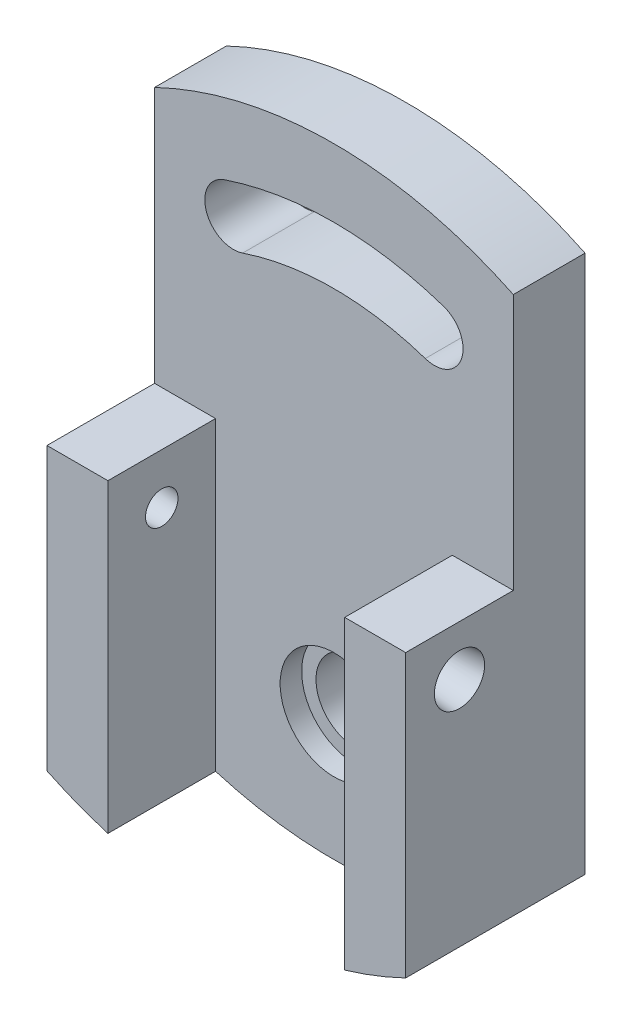
ISO-10303-21;
HEADER;
FILE_DESCRIPTION(('STEP AP214'),'2;1');
FILE_NAME('part.step','',(''),(''),'','','');
FILE_SCHEMA(('AUTOMOTIVE_DESIGN { 1 0 10303 214 1 1 1 1 }'));
ENDSEC;
DATA;
#1=APPLICATION_CONTEXT('core data for automotive mechanical design processes');
#2=APPLICATION_PROTOCOL_DEFINITION('international standard','automotive_design',2000,#1);
#3=PRODUCT_CONTEXT('',#1,'mechanical');
#4=PRODUCT('Part','Part','',(#3));
#5=PRODUCT_RELATED_PRODUCT_CATEGORY('part','',(#4));
#6=PRODUCT_DEFINITION_FORMATION('','',#4);
#7=PRODUCT_DEFINITION_CONTEXT('part definition',#1,'design');
#8=PRODUCT_DEFINITION('design','',#6,#7);
#9=PRODUCT_DEFINITION_SHAPE('','',#8);
#10=(LENGTH_UNIT() NAMED_UNIT(*) SI_UNIT(.MILLI.,.METRE.));
#11=(NAMED_UNIT(*) PLANE_ANGLE_UNIT() SI_UNIT($,.RADIAN.));
#12=(NAMED_UNIT(*) SI_UNIT($,.STERADIAN.) SOLID_ANGLE_UNIT());
#13=UNCERTAINTY_MEASURE_WITH_UNIT(LENGTH_MEASURE(1.E-05),#10,'distance_accuracy_value','');
#14=(GEOMETRIC_REPRESENTATION_CONTEXT(3) GLOBAL_UNCERTAINTY_ASSIGNED_CONTEXT((#13)) GLOBAL_UNIT_ASSIGNED_CONTEXT((#10,
#11,#12)) REPRESENTATION_CONTEXT('',''));
#15=CARTESIAN_POINT('',(0.,0.,0.));
#16=DIRECTION('',(0.,0.,1.));
#17=DIRECTION('',(1.,0.,0.));
#18=AXIS2_PLACEMENT_3D('',#15,#16,#17);
#19=CARTESIAN_POINT('',(0.,17.1231517720798,10.));
#20=DIRECTION('',(0.,0.,1.));
#21=DIRECTION('',(1.,0.,0.));
#22=AXIS2_PLACEMENT_3D('',#19,#20,#21);
#23=PLANE('',#22);
#24=CARTESIAN_POINT('',(28.,43.4266144584568,10.));
#25=DIRECTION('',(0.,0.,1.));
#26=DIRECTION('',(1.,0.,0.));
#27=AXIS2_PLACEMENT_3D('',#24,#25,#26);
#28=CIRCLE('',#27,8.00000000000001);
#29=CARTESIAN_POINT('',(25.4545454545455,35.8423767804153,10.));
#30=VERTEX_POINT('',#29);
#31=CARTESIAN_POINT('',(30.5454545454546,51.0108521364984,10.));
#32=VERTEX_POINT('',#31);
#33=EDGE_CURVE('E197',#30,#32,#28,.T.);
#34=ORIENTED_EDGE('',*,*,#33,.F.);
#35=CARTESIAN_POINT('',(0.,-40.,10.));
#36=DIRECTION('',(0.,0.,-1.));
#37=DIRECTION('',(1.,0.,0.));
#38=AXIS2_PLACEMENT_3D('',#35,#36,#37);
#39=CIRCLE('',#38,80.);
#40=CARTESIAN_POINT('',(-25.4545454545455,35.8423767804153,10.));
#41=VERTEX_POINT('',#40);
#42=EDGE_CURVE('E201',#41,#30,#39,.T.);
#43=ORIENTED_EDGE('',*,*,#42,.F.);
#44=CARTESIAN_POINT('',(-28.,43.4266144584568,10.));
#45=DIRECTION('',(0.,0.,1.));
#46=DIRECTION('',(1.,0.,0.));
#47=AXIS2_PLACEMENT_3D('',#44,#45,#46);
#48=CIRCLE('',#47,8.00000000000001);
#49=CARTESIAN_POINT('',(-30.5454545454545,51.0108521364984,10.));
#50=VERTEX_POINT('',#49);
#51=EDGE_CURVE('E213',#50,#41,#48,.T.);
#52=ORIENTED_EDGE('',*,*,#51,.F.);
#53=CARTESIAN_POINT('',(0.,-40.,10.));
#54=DIRECTION('',(0.,0.,1.));
#55=DIRECTION('',(1.,0.,0.));
#56=AXIS2_PLACEMENT_3D('',#53,#54,#55);
#57=CIRCLE('',#56,96.);
#58=EDGE_CURVE('E215',#32,#50,#57,.T.);
#59=ORIENTED_EDGE('',*,*,#58,.F.);
#60=EDGE_LOOP('',(#34,#43,#52,#59));
#61=FACE_BOUND('',#60,.T.);
#62=CARTESIAN_POINT('',(0.,-62.8768482279202,10.));
#63=DIRECTION('',(0.,0.,1.));
#64=DIRECTION('',(1.,0.,0.));
#65=AXIS2_PLACEMENT_3D('',#62,#63,#64);
#66=CIRCLE('',#65,15.);
#67=CARTESIAN_POINT('',(15.,-62.8768482279202,10.));
#68=VERTEX_POINT('',#67);
#69=EDGE_CURVE('E236',#68,#68,#66,.T.);
#70=ORIENTED_EDGE('',*,*,#69,.F.);
#71=EDGE_LOOP('',(#70));
#72=FACE_BOUND('',#71,.T.);
#73=DIRECTION('',(0.,-1.,0.));
#74=VECTOR('',#73,1.);
#75=CARTESIAN_POINT('',(33.,0.,10.));
#76=LINE('',#75,#74);
#77=CARTESIAN_POINT('',(33.,-7.87684822792019,10.));
#78=VERTEX_POINT('',#77);
#79=CARTESIAN_POINT('',(33.,-93.0403630592835,10.));
#80=VERTEX_POINT('',#79);
#81=EDGE_CURVE('E58',#78,#80,#76,.T.);
#82=ORIENTED_EDGE('',*,*,#81,.F.);
#83=DIRECTION('',(-1.,0.,0.));
#84=VECTOR('',#83,1.);
#85=CARTESIAN_POINT('',(0.,-7.87684822792019,10.));
#86=LINE('',#85,#84);
#87=CARTESIAN_POINT('',(50.,-7.87684822792019,10.));
#88=VERTEX_POINT('',#87);
#89=EDGE_CURVE('E317',#88,#78,#86,.T.);
#90=ORIENTED_EDGE('',*,*,#89,.F.);
#91=DIRECTION('',(0.,1.,0.));
#92=VECTOR('',#91,1.);
#93=CARTESIAN_POINT('',(50.,-86.4384241139601,10.));
#94=LINE('',#93,#92);
#95=CARTESIAN_POINT('',(50.,63.5615758860399,10.));
#96=VERTEX_POINT('',#95);
#97=EDGE_CURVE('E170',#88,#96,#94,.T.);
#98=ORIENTED_EDGE('',*,*,#97,.T.);
#99=CARTESIAN_POINT('',(0.,-40.,10.));
#100=DIRECTION('',(0.,0.,1.));
#101=DIRECTION('',(-1.,0.,0.));
#102=AXIS2_PLACEMENT_3D('',#99,#100,#101);
#103=CIRCLE('',#102,115.);
#104=CARTESIAN_POINT('',(-50.,63.5615758860399,10.));
#105=VERTEX_POINT('',#104);
#106=EDGE_CURVE('E245',#96,#105,#103,.T.);
#107=ORIENTED_EDGE('',*,*,#106,.T.);
#108=DIRECTION('',(0.,-1.,0.));
#109=VECTOR('',#108,1.);
#110=CARTESIAN_POINT('',(-50.,-86.4384241139601,10.));
#111=LINE('',#110,#109);
#112=CARTESIAN_POINT('',(-50.,-7.87684822792019,10.));
#113=VERTEX_POINT('',#112);
#114=EDGE_CURVE('E242',#105,#113,#111,.T.);
#115=ORIENTED_EDGE('',*,*,#114,.T.);
#116=DIRECTION('',(1.,0.,0.));
#117=VECTOR('',#116,1.);
#118=CARTESIAN_POINT('',(0.,-7.87684822792019,10.));
#119=LINE('',#118,#117);
#120=CARTESIAN_POINT('',(-33.,-7.87684822792019,10.));
#121=VERTEX_POINT('',#120);
#122=EDGE_CURVE('E167',#113,#121,#119,.T.);
#123=ORIENTED_EDGE('',*,*,#122,.T.);
#124=DIRECTION('',(0.,-1.,0.));
#125=VECTOR('',#124,1.);
#126=CARTESIAN_POINT('',(-33.,0.,10.));
#127=LINE('',#126,#125);
#128=CARTESIAN_POINT('',(-33.,-93.0403630592835,10.));
#129=VERTEX_POINT('',#128);
#130=EDGE_CURVE('E166',#121,#129,#127,.T.);
#131=ORIENTED_EDGE('',*,*,#130,.T.);
#132=CARTESIAN_POINT('',(0.,17.1231517720798,10.));
#133=DIRECTION('',(0.,0.,1.));
#134=DIRECTION('',(1.,0.,0.));
#135=AXIS2_PLACEMENT_3D('',#132,#133,#134);
#136=CIRCLE('',#135,115.);
#137=EDGE_CURVE('E63',#129,#80,#136,.T.);
#138=ORIENTED_EDGE('',*,*,#137,.T.);
#139=EDGE_LOOP('',(#82,#90,#98,#107,#115,#123,#131,#138));
#140=FACE_BOUND('',#139,.T.);
#141=ADVANCED_FACE('F43',(#61,#72,#140),#23,.T.);
#142=CARTESIAN_POINT('',(0.,17.1231517720798,10.));
#143=DIRECTION('',(0.,0.,-1.));
#144=DIRECTION('',(-1.,0.,0.));
#145=AXIS2_PLACEMENT_3D('',#142,#143,#144);
#146=CYLINDRICAL_SURFACE('',#145,115.);
#147=CARTESIAN_POINT('',(0.,17.1231517720798,-10.));
#148=DIRECTION('',(0.,0.,1.));
#149=DIRECTION('',(1.,0.,0.));
#150=AXIS2_PLACEMENT_3D('',#147,#148,#149);
#151=CIRCLE('',#150,115.);
#152=CARTESIAN_POINT('',(-50.,-86.4384241139601,-10.));
#153=VERTEX_POINT('',#152);
#154=CARTESIAN_POINT('',(50.,-86.4384241139601,-10.));
#155=VERTEX_POINT('',#154);
#156=EDGE_CURVE('E232',#153,#155,#151,.T.);
#157=ORIENTED_EDGE('',*,*,#156,.T.);
#158=DIRECTION('',(0.,0.,-1.));
#159=VECTOR('',#158,1.);
#160=CARTESIAN_POINT('',(50.,-86.4384241139601,10.));
#161=LINE('',#160,#159);
#162=CARTESIAN_POINT('',(50.,-86.4384241139601,40.));
#163=VERTEX_POINT('',#162);
#164=EDGE_CURVE('E12',#163,#155,#161,.T.);
#165=ORIENTED_EDGE('',*,*,#164,.F.);
#166=CARTESIAN_POINT('',(0.,17.1231517720798,40.));
#167=DIRECTION('',(0.,0.,1.));
#168=DIRECTION('',(1.,0.,0.));
#169=AXIS2_PLACEMENT_3D('',#166,#167,#168);
#170=CIRCLE('',#169,115.);
#171=CARTESIAN_POINT('',(33.,-93.0403630592835,40.));
#172=VERTEX_POINT('',#171);
#173=EDGE_CURVE('E162',#172,#163,#170,.T.);
#174=ORIENTED_EDGE('',*,*,#173,.F.);
#175=DIRECTION('',(0.,0.,-1.));
#176=VECTOR('',#175,1.);
#177=CARTESIAN_POINT('',(33.,-93.0403630592835,40.));
#178=LINE('',#177,#176);
#179=EDGE_CURVE('E175',#172,#80,#178,.T.);
#180=ORIENTED_EDGE('',*,*,#179,.T.);
#181=ORIENTED_EDGE('',*,*,#137,.F.);
#182=DIRECTION('',(0.,0.,-1.));
#183=VECTOR('',#182,1.);
#184=CARTESIAN_POINT('',(-33.,-93.0403630592835,40.));
#185=LINE('',#184,#183);
#186=CARTESIAN_POINT('',(-33.,-93.0403630592835,40.));
#187=VERTEX_POINT('',#186);
#188=EDGE_CURVE('E187',#187,#129,#185,.T.);
#189=ORIENTED_EDGE('',*,*,#188,.F.);
#190=CARTESIAN_POINT('',(0.,17.1231517720798,40.));
#191=DIRECTION('',(0.,0.,1.));
#192=DIRECTION('',(1.,0.,0.));
#193=AXIS2_PLACEMENT_3D('',#190,#191,#192);
#194=CIRCLE('',#193,115.);
#195=CARTESIAN_POINT('',(-50.,-86.4384241139601,40.));
#196=VERTEX_POINT('',#195);
#197=EDGE_CURVE('E184',#196,#187,#194,.T.);
#198=ORIENTED_EDGE('',*,*,#197,.F.);
#199=DIRECTION('',(0.,0.,-1.));
#200=VECTOR('',#199,1.);
#201=CARTESIAN_POINT('',(-50.,-86.4384241139601,10.));
#202=LINE('',#201,#200);
#203=EDGE_CURVE('E250',#196,#153,#202,.T.);
#204=ORIENTED_EDGE('',*,*,#203,.T.);
#205=EDGE_LOOP('',(#157,#165,#174,#180,#181,#189,#198,#204));
#206=FACE_BOUND('',#205,.T.);
#207=ADVANCED_FACE('F44',(#206),#146,.T.);
#208=CARTESIAN_POINT('',(50.,-86.4384241139601,10.));
#209=DIRECTION('',(-1.,0.,0.));
#210=DIRECTION('',(0.,0.,1.));
#211=AXIS2_PLACEMENT_3D('',#208,#209,#210);
#212=PLANE('',#211);
#213=CARTESIAN_POINT('',(50.,-21.8768482279202,25.));
#214=DIRECTION('',(1.,0.,0.));
#215=DIRECTION('',(0.,0.,-1.));
#216=AXIS2_PLACEMENT_3D('',#213,#214,#215);
#217=CIRCLE('',#216,7.);
#218=CARTESIAN_POINT('',(50.,-18.0410436799808,30.8554763657628));
#219=VERTEX_POINT('',#218);
#220=EDGE_CURVE('E310',#219,#219,#217,.T.);
#221=ORIENTED_EDGE('',*,*,#220,.F.);
#222=EDGE_LOOP('',(#221));
#223=FACE_BOUND('',#222,.T.);
#224=DIRECTION('',(0.,1.,0.));
#225=VECTOR('',#224,1.);
#226=CARTESIAN_POINT('',(50.,-86.4384241139601,-10.));
#227=LINE('',#226,#225);
#228=CARTESIAN_POINT('',(50.,63.5615758860399,-10.));
#229=VERTEX_POINT('',#228);
#230=EDGE_CURVE('E249',#155,#229,#227,.T.);
#231=ORIENTED_EDGE('',*,*,#230,.T.);
#232=DIRECTION('',(0.,0.,-1.));
#233=VECTOR('',#232,1.);
#234=CARTESIAN_POINT('',(50.,63.5615758860399,10.));
#235=LINE('',#234,#233);
#236=EDGE_CURVE('E55',#96,#229,#235,.T.);
#237=ORIENTED_EDGE('',*,*,#236,.F.);
#238=ORIENTED_EDGE('',*,*,#97,.F.);
#239=DIRECTION('',(0.,0.,-1.));
#240=VECTOR('',#239,1.);
#241=CARTESIAN_POINT('',(50.,-7.87684822792019,40.));
#242=LINE('',#241,#240);
#243=CARTESIAN_POINT('',(50.,-7.87684822792019,40.));
#244=VERTEX_POINT('',#243);
#245=EDGE_CURVE('E148',#244,#88,#242,.T.);
#246=ORIENTED_EDGE('',*,*,#245,.F.);
#247=DIRECTION('',(0.,1.,0.));
#248=VECTOR('',#247,1.);
#249=CARTESIAN_POINT('',(50.,0.,40.));
#250=LINE('',#249,#248);
#251=EDGE_CURVE('E156',#163,#244,#250,.T.);
#252=ORIENTED_EDGE('',*,*,#251,.F.);
#253=ORIENTED_EDGE('',*,*,#164,.T.);
#254=EDGE_LOOP('',(#231,#237,#238,#246,#252,#253));
#255=FACE_BOUND('',#254,.T.);
#256=ADVANCED_FACE('F164',(#223,#255),#212,.F.);
#257=CARTESIAN_POINT('',(0.,-40.,10.));
#258=DIRECTION('',(0.,0.,-1.));
#259=DIRECTION('',(-1.,0.,0.));
#260=AXIS2_PLACEMENT_3D('',#257,#258,#259);
#261=CYLINDRICAL_SURFACE('',#260,115.);
#262=CARTESIAN_POINT('',(0.,-40.,-10.));
#263=DIRECTION('',(0.,0.,1.));
#264=DIRECTION('',(-1.,0.,0.));
#265=AXIS2_PLACEMENT_3D('',#262,#263,#264);
#266=CIRCLE('',#265,115.);
#267=CARTESIAN_POINT('',(-50.,63.5615758860399,-10.));
#268=VERTEX_POINT('',#267);
#269=EDGE_CURVE('E255',#229,#268,#266,.T.);
#270=ORIENTED_EDGE('',*,*,#269,.T.);
#271=DIRECTION('',(0.,0.,-1.));
#272=VECTOR('',#271,1.);
#273=CARTESIAN_POINT('',(-50.,63.5615758860399,10.));
#274=LINE('',#273,#272);
#275=EDGE_CURVE('E260',#105,#268,#274,.T.);
#276=ORIENTED_EDGE('',*,*,#275,.F.);
#277=ORIENTED_EDGE('',*,*,#106,.F.);
#278=ORIENTED_EDGE('',*,*,#236,.T.);
#279=EDGE_LOOP('',(#270,#276,#277,#278));
#280=FACE_BOUND('',#279,.T.);
#281=ADVANCED_FACE('F298',(#280),#261,.T.);
#282=CARTESIAN_POINT('',(-50.,-86.4384241139601,10.));
#283=DIRECTION('',(1.,0.,0.));
#284=DIRECTION('',(0.,0.,-1.));
#285=AXIS2_PLACEMENT_3D('',#282,#283,#284);
#286=PLANE('',#285);
#287=CARTESIAN_POINT('',(-50.,-21.8768482279202,25.));
#288=DIRECTION('',(-1.,0.,0.));
#289=DIRECTION('',(0.,0.,1.));
#290=AXIS2_PLACEMENT_3D('',#287,#288,#289);
#291=CIRCLE('',#290,6.);
#292=CARTESIAN_POINT('',(-50.,-27.8608007953017,25.4385335464111));
#293=VERTEX_POINT('',#292);
#294=EDGE_CURVE('E307',#293,#293,#291,.T.);
#295=ORIENTED_EDGE('',*,*,#294,.F.);
#296=EDGE_LOOP('',(#295));
#297=FACE_BOUND('',#296,.T.);
#298=DIRECTION('',(0.,-1.,0.));
#299=VECTOR('',#298,1.);
#300=CARTESIAN_POINT('',(-50.,-86.4384241139601,-10.));
#301=LINE('',#300,#299);
#302=EDGE_CURVE('E239',#268,#153,#301,.T.);
#303=ORIENTED_EDGE('',*,*,#302,.T.);
#304=ORIENTED_EDGE('',*,*,#203,.F.);
#305=DIRECTION('',(0.,-1.,0.));
#306=VECTOR('',#305,1.);
#307=CARTESIAN_POINT('',(-50.,0.,40.));
#308=LINE('',#307,#306);
#309=CARTESIAN_POINT('',(-50.,-7.87684822792019,40.));
#310=VERTEX_POINT('',#309);
#311=EDGE_CURVE('E185',#310,#196,#308,.T.);
#312=ORIENTED_EDGE('',*,*,#311,.F.);
#313=DIRECTION('',(0.,0.,-1.));
#314=VECTOR('',#313,1.);
#315=CARTESIAN_POINT('',(-50.,-7.87684822792019,40.));
#316=LINE('',#315,#314);
#317=EDGE_CURVE('E192',#310,#113,#316,.T.);
#318=ORIENTED_EDGE('',*,*,#317,.T.);
#319=ORIENTED_EDGE('',*,*,#114,.F.);
#320=ORIENTED_EDGE('',*,*,#275,.T.);
#321=EDGE_LOOP('',(#303,#304,#312,#318,#319,#320));
#322=FACE_BOUND('',#321,.T.);
#323=ADVANCED_FACE('F292',(#297,#322),#286,.F.);
#324=CARTESIAN_POINT('',(0.,17.1231517720798,-10.));
#325=DIRECTION('',(0.,0.,1.));
#326=DIRECTION('',(1.,0.,0.));
#327=AXIS2_PLACEMENT_3D('',#324,#325,#326);
#328=PLANE('',#327);
#329=CARTESIAN_POINT('',(0.,-40.,-10.));
#330=DIRECTION('',(0.,0.,-1.));
#331=DIRECTION('',(1.,0.,0.));
#332=AXIS2_PLACEMENT_3D('',#329,#330,#331);
#333=CIRCLE('',#332,80.);
#334=CARTESIAN_POINT('',(-25.4545454545455,35.8423767804153,-10.));
#335=VERTEX_POINT('',#334);
#336=CARTESIAN_POINT('',(25.4545454545455,35.8423767804153,-10.));
#337=VERTEX_POINT('',#336);
#338=EDGE_CURVE('E210',#335,#337,#333,.T.);
#339=ORIENTED_EDGE('',*,*,#338,.T.);
#340=CARTESIAN_POINT('',(28.,43.4266144584568,-10.));
#341=DIRECTION('',(0.,0.,1.));
#342=DIRECTION('',(1.,0.,0.));
#343=AXIS2_PLACEMENT_3D('',#340,#341,#342);
#344=CIRCLE('',#343,8.00000000000001);
#345=CARTESIAN_POINT('',(30.5454545454546,51.0108521364984,-10.));
#346=VERTEX_POINT('',#345);
#347=EDGE_CURVE('E200',#337,#346,#344,.T.);
#348=ORIENTED_EDGE('',*,*,#347,.T.);
#349=CARTESIAN_POINT('',(0.,-40.,-10.));
#350=DIRECTION('',(0.,0.,1.));
#351=DIRECTION('',(1.,0.,0.));
#352=AXIS2_PLACEMENT_3D('',#349,#350,#351);
#353=CIRCLE('',#352,96.);
#354=CARTESIAN_POINT('',(-30.5454545454545,51.0108521364984,-10.));
#355=VERTEX_POINT('',#354);
#356=EDGE_CURVE('E198',#346,#355,#353,.T.);
#357=ORIENTED_EDGE('',*,*,#356,.T.);
#358=CARTESIAN_POINT('',(-28.,43.4266144584568,-10.));
#359=DIRECTION('',(0.,0.,1.));
#360=DIRECTION('',(1.,0.,0.));
#361=AXIS2_PLACEMENT_3D('',#358,#359,#360);
#362=CIRCLE('',#361,8.00000000000001);
#363=EDGE_CURVE('E203',#355,#335,#362,.T.);
#364=ORIENTED_EDGE('',*,*,#363,.T.);
#365=EDGE_LOOP('',(#339,#348,#357,#364));
#366=FACE_BOUND('',#365,.T.);
#367=CARTESIAN_POINT('',(0.,-62.8768482279202,-10.));
#368=DIRECTION('',(0.,0.,1.));
#369=DIRECTION('',(1.,0.,0.));
#370=AXIS2_PLACEMENT_3D('',#367,#368,#369);
#371=CIRCLE('',#370,11.);
#372=CARTESIAN_POINT('',(11.,-62.8768482279202,-10.));
#373=VERTEX_POINT('',#372);
#374=EDGE_CURVE('E225',#373,#373,#371,.T.);
#375=ORIENTED_EDGE('',*,*,#374,.T.);
#376=EDGE_LOOP('',(#375));
#377=FACE_BOUND('',#376,.T.);
#378=ORIENTED_EDGE('',*,*,#156,.F.);
#379=ORIENTED_EDGE('',*,*,#302,.F.);
#380=ORIENTED_EDGE('',*,*,#269,.F.);
#381=ORIENTED_EDGE('',*,*,#230,.F.);
#382=EDGE_LOOP('',(#378,#379,#380,#381));
#383=FACE_BOUND('',#382,.T.);
#384=ADVANCED_FACE('F277',(#366,#377,#383),#328,.F.);
#385=CARTESIAN_POINT('',(0.,-62.8768482279202,4.));
#386=DIRECTION('',(0.,0.,1.));
#387=DIRECTION('',(1.,0.,0.));
#388=AXIS2_PLACEMENT_3D('',#385,#386,#387);
#389=CYLINDRICAL_SURFACE('',#388,15.);
#390=CARTESIAN_POINT('',(0.,-62.8768482279202,4.));
#391=DIRECTION('',(0.,0.,1.));
#392=DIRECTION('',(1.,0.,0.));
#393=AXIS2_PLACEMENT_3D('',#390,#391,#392);
#394=CIRCLE('',#393,15.);
#395=CARTESIAN_POINT('',(15.,-62.8768482279202,4.));
#396=VERTEX_POINT('',#395);
#397=EDGE_CURVE('E235',#396,#396,#394,.T.);
#398=ORIENTED_EDGE('',*,*,#397,.F.);
#399=EDGE_LOOP('',(#398));
#400=FACE_BOUND('',#399,.T.);
#401=ORIENTED_EDGE('',*,*,#69,.T.);
#402=EDGE_LOOP('',(#401));
#403=FACE_BOUND('',#402,.T.);
#404=ADVANCED_FACE('F269',(#400,#403),#389,.F.);
#405=CARTESIAN_POINT('',(0.,-62.8768482279202,4.));
#406=DIRECTION('',(0.,0.,1.));
#407=DIRECTION('',(1.,0.,0.));
#408=AXIS2_PLACEMENT_3D('',#405,#406,#407);
#409=PLANE('',#408);
#410=CARTESIAN_POINT('',(0.,-62.8768482279202,4.));
#411=DIRECTION('',(0.,0.,1.));
#412=DIRECTION('',(1.,0.,0.));
#413=AXIS2_PLACEMENT_3D('',#410,#411,#412);
#414=CIRCLE('',#413,11.);
#415=CARTESIAN_POINT('',(11.,-62.8768482279202,4.));
#416=VERTEX_POINT('',#415);
#417=EDGE_CURVE('E233',#416,#416,#414,.T.);
#418=ORIENTED_EDGE('',*,*,#417,.F.);
#419=EDGE_LOOP('',(#418));
#420=FACE_BOUND('',#419,.T.);
#421=ORIENTED_EDGE('',*,*,#397,.T.);
#422=EDGE_LOOP('',(#421));
#423=FACE_BOUND('',#422,.T.);
#424=ADVANCED_FACE('F270',(#420,#423),#409,.T.);
#425=CARTESIAN_POINT('',(0.,-62.8768482279202,-10.));
#426=DIRECTION('',(0.,0.,1.));
#427=DIRECTION('',(1.,0.,0.));
#428=AXIS2_PLACEMENT_3D('',#425,#426,#427);
#429=CYLINDRICAL_SURFACE('',#428,11.);
#430=ORIENTED_EDGE('',*,*,#417,.T.);
#431=EDGE_LOOP('',(#430));
#432=FACE_BOUND('',#431,.T.);
#433=ORIENTED_EDGE('',*,*,#374,.F.);
#434=EDGE_LOOP('',(#433));
#435=FACE_BOUND('',#434,.T.);
#436=ADVANCED_FACE('F261',(#432,#435),#429,.F.);
#437=CARTESIAN_POINT('',(28.,43.4266144584568,-10.));
#438=DIRECTION('',(0.,0.,1.));
#439=DIRECTION('',(1.,0.,0.));
#440=AXIS2_PLACEMENT_3D('',#437,#438,#439);
#441=CYLINDRICAL_SURFACE('',#440,8.00000000000001);
#442=ORIENTED_EDGE('',*,*,#33,.T.);
#443=DIRECTION('',(0.,0.,1.));
#444=VECTOR('',#443,1.);
#445=CARTESIAN_POINT('',(30.5454545454546,51.0108521364984,-10.));
#446=LINE('',#445,#444);
#447=EDGE_CURVE('E208',#346,#32,#446,.T.);
#448=ORIENTED_EDGE('',*,*,#447,.F.);
#449=ORIENTED_EDGE('',*,*,#347,.F.);
#450=DIRECTION('',(0.,0.,1.));
#451=VECTOR('',#450,1.);
#452=CARTESIAN_POINT('',(25.4545454545455,35.8423767804153,-10.));
#453=LINE('',#452,#451);
#454=EDGE_CURVE('E218',#337,#30,#453,.T.);
#455=ORIENTED_EDGE('',*,*,#454,.T.);
#456=EDGE_LOOP('',(#442,#448,#449,#455));
#457=FACE_BOUND('',#456,.T.);
#458=ADVANCED_FACE('F358',(#457),#441,.F.);
#459=CARTESIAN_POINT('',(0.,-40.,-10.));
#460=DIRECTION('',(0.,0.,1.));
#461=DIRECTION('',(1.,0.,0.));
#462=AXIS2_PLACEMENT_3D('',#459,#460,#461);
#463=CYLINDRICAL_SURFACE('',#462,80.);
#464=ORIENTED_EDGE('',*,*,#42,.T.);
#465=ORIENTED_EDGE('',*,*,#454,.F.);
#466=ORIENTED_EDGE('',*,*,#338,.F.);
#467=DIRECTION('',(0.,0.,1.));
#468=VECTOR('',#467,1.);
#469=CARTESIAN_POINT('',(-25.4545454545455,35.8423767804153,-10.));
#470=LINE('',#469,#468);
#471=EDGE_CURVE('E222',#335,#41,#470,.T.);
#472=ORIENTED_EDGE('',*,*,#471,.T.);
#473=EDGE_LOOP('',(#464,#465,#466,#472));
#474=FACE_BOUND('',#473,.T.);
#475=ADVANCED_FACE('F355',(#474),#463,.T.);
#476=CARTESIAN_POINT('',(-28.,43.4266144584568,-10.));
#477=DIRECTION('',(0.,0.,1.));
#478=DIRECTION('',(1.,0.,0.));
#479=AXIS2_PLACEMENT_3D('',#476,#477,#478);
#480=CYLINDRICAL_SURFACE('',#479,8.00000000000001);
#481=ORIENTED_EDGE('',*,*,#51,.T.);
#482=ORIENTED_EDGE('',*,*,#471,.F.);
#483=ORIENTED_EDGE('',*,*,#363,.F.);
#484=DIRECTION('',(0.,0.,1.));
#485=VECTOR('',#484,1.);
#486=CARTESIAN_POINT('',(-30.5454545454545,51.0108521364984,-10.));
#487=LINE('',#486,#485);
#488=EDGE_CURVE('E224',#355,#50,#487,.T.);
#489=ORIENTED_EDGE('',*,*,#488,.T.);
#490=EDGE_LOOP('',(#481,#482,#483,#489));
#491=FACE_BOUND('',#490,.T.);
#492=ADVANCED_FACE('F354',(#491),#480,.F.);
#493=CARTESIAN_POINT('',(0.,-40.,-10.));
#494=DIRECTION('',(0.,0.,1.));
#495=DIRECTION('',(1.,0.,0.));
#496=AXIS2_PLACEMENT_3D('',#493,#494,#495);
#497=CYLINDRICAL_SURFACE('',#496,96.);
#498=ORIENTED_EDGE('',*,*,#58,.T.);
#499=ORIENTED_EDGE('',*,*,#488,.F.);
#500=ORIENTED_EDGE('',*,*,#356,.F.);
#501=ORIENTED_EDGE('',*,*,#447,.T.);
#502=EDGE_LOOP('',(#498,#499,#500,#501));
#503=FACE_BOUND('',#502,.T.);
#504=ADVANCED_FACE('F348',(#503),#497,.F.);
#505=CARTESIAN_POINT('',(-33.,0.,40.));
#506=DIRECTION('',(1.,0.,0.));
#507=DIRECTION('',(0.,1.,0.));
#508=AXIS2_PLACEMENT_3D('',#505,#506,#507);
#509=PLANE('',#508);
#510=CARTESIAN_POINT('',(-33.,-21.8768482279202,25.));
#511=DIRECTION('',(-1.,0.,0.));
#512=DIRECTION('',(0.,0.,1.));
#513=AXIS2_PLACEMENT_3D('',#510,#511,#512);
#514=CIRCLE('',#513,4.52368501413102);
#515=CARTESIAN_POINT('',(-33.,-26.1914420856972,26.3594138257009));
#516=VERTEX_POINT('',#515);
#517=EDGE_CURVE('E313',#516,#516,#514,.F.);
#518=ORIENTED_EDGE('',*,*,#517,.F.);
#519=EDGE_LOOP('',(#518));
#520=FACE_BOUND('',#519,.T.);
#521=ORIENTED_EDGE('',*,*,#130,.F.);
#522=DIRECTION('',(0.,0.,-1.));
#523=VECTOR('',#522,1.);
#524=CARTESIAN_POINT('',(-33.,-7.87684822792019,40.));
#525=LINE('',#524,#523);
#526=CARTESIAN_POINT('',(-33.,-7.87684822792019,40.));
#527=VERTEX_POINT('',#526);
#528=EDGE_CURVE('E194',#527,#121,#525,.T.);
#529=ORIENTED_EDGE('',*,*,#528,.F.);
#530=DIRECTION('',(0.,-1.,0.));
#531=VECTOR('',#530,1.);
#532=CARTESIAN_POINT('',(-33.,0.,40.));
#533=LINE('',#532,#531);
#534=EDGE_CURVE('E176',#527,#187,#533,.T.);
#535=ORIENTED_EDGE('',*,*,#534,.T.);
#536=ORIENTED_EDGE('',*,*,#188,.T.);
#537=EDGE_LOOP('',(#521,#529,#535,#536));
#538=FACE_BOUND('',#537,.T.);
#539=ADVANCED_FACE('F350',(#520,#538),#509,.T.);
#540=CARTESIAN_POINT('',(0.,-7.87684822792019,40.));
#541=DIRECTION('',(0.,1.,0.));
#542=DIRECTION('',(0.,0.,1.));
#543=AXIS2_PLACEMENT_3D('',#540,#541,#542);
#544=PLANE('',#543);
#545=ORIENTED_EDGE('',*,*,#122,.F.);
#546=ORIENTED_EDGE('',*,*,#317,.F.);
#547=DIRECTION('',(1.,0.,0.));
#548=VECTOR('',#547,1.);
#549=CARTESIAN_POINT('',(0.,-7.87684822792019,40.));
#550=LINE('',#549,#548);
#551=EDGE_CURVE('E177',#310,#527,#550,.T.);
#552=ORIENTED_EDGE('',*,*,#551,.T.);
#553=ORIENTED_EDGE('',*,*,#528,.T.);
#554=EDGE_LOOP('',(#545,#546,#552,#553));
#555=FACE_BOUND('',#554,.T.);
#556=ADVANCED_FACE('F344',(#555),#544,.T.);
#557=CARTESIAN_POINT('',(0.,0.,40.));
#558=DIRECTION('',(0.,0.,1.));
#559=DIRECTION('',(1.,0.,0.));
#560=AXIS2_PLACEMENT_3D('',#557,#558,#559);
#561=PLANE('',#560);
#562=ORIENTED_EDGE('',*,*,#534,.F.);
#563=ORIENTED_EDGE('',*,*,#551,.F.);
#564=ORIENTED_EDGE('',*,*,#311,.T.);
#565=ORIENTED_EDGE('',*,*,#197,.T.);
#566=EDGE_LOOP('',(#562,#563,#564,#565));
#567=FACE_BOUND('',#566,.T.);
#568=ADVANCED_FACE('F337',(#567),#561,.T.);
#569=CARTESIAN_POINT('',(0.,-7.87684822792019,40.));
#570=DIRECTION('',(0.,-1.,0.));
#571=DIRECTION('',(0.,0.,-1.));
#572=AXIS2_PLACEMENT_3D('',#569,#570,#571);
#573=PLANE('',#572);
#574=ORIENTED_EDGE('',*,*,#89,.T.);
#575=DIRECTION('',(0.,0.,-1.));
#576=VECTOR('',#575,1.);
#577=CARTESIAN_POINT('',(33.,-7.87684822792019,40.));
#578=LINE('',#577,#576);
#579=CARTESIAN_POINT('',(33.,-7.87684822792019,40.));
#580=VERTEX_POINT('',#579);
#581=EDGE_CURVE('E155',#580,#78,#578,.T.);
#582=ORIENTED_EDGE('',*,*,#581,.F.);
#583=DIRECTION('',(-1.,0.,0.));
#584=VECTOR('',#583,1.);
#585=CARTESIAN_POINT('',(0.,-7.87684822792019,40.));
#586=LINE('',#585,#584);
#587=EDGE_CURVE('E147',#244,#580,#586,.T.);
#588=ORIENTED_EDGE('',*,*,#587,.F.);
#589=ORIENTED_EDGE('',*,*,#245,.T.);
#590=EDGE_LOOP('',(#574,#582,#588,#589));
#591=FACE_BOUND('',#590,.T.);
#592=ADVANCED_FACE('F149',(#591),#573,.F.);
#593=CARTESIAN_POINT('',(33.,0.,40.));
#594=DIRECTION('',(1.,0.,0.));
#595=DIRECTION('',(0.,1.,0.));
#596=AXIS2_PLACEMENT_3D('',#593,#594,#595);
#597=PLANE('',#596);
#598=CARTESIAN_POINT('',(33.,-21.8768482279202,25.));
#599=DIRECTION('',(-1.,0.,0.));
#600=DIRECTION('',(0.,0.,1.));
#601=AXIS2_PLACEMENT_3D('',#598,#599,#600);
#602=CIRCLE('',#601,5.38922314504359);
#603=CARTESIAN_POINT('',(33.,-19.7104023895853,29.9345960864731));
#604=VERTEX_POINT('',#603);
#605=EDGE_CURVE('E50',#604,#604,#602,.F.);
#606=ORIENTED_EDGE('',*,*,#605,.T.);
#607=EDGE_LOOP('',(#606));
#608=FACE_BOUND('',#607,.T.);
#609=ORIENTED_EDGE('',*,*,#81,.T.);
#610=ORIENTED_EDGE('',*,*,#179,.F.);
#611=DIRECTION('',(0.,-1.,0.));
#612=VECTOR('',#611,1.);
#613=CARTESIAN_POINT('',(33.,0.,40.));
#614=LINE('',#613,#612);
#615=EDGE_CURVE('E153',#580,#172,#614,.T.);
#616=ORIENTED_EDGE('',*,*,#615,.F.);
#617=ORIENTED_EDGE('',*,*,#581,.T.);
#618=EDGE_LOOP('',(#609,#610,#616,#617));
#619=FACE_BOUND('',#618,.T.);
#620=ADVANCED_FACE('F323',(#608,#619),#597,.F.);
#621=CARTESIAN_POINT('',(0.,0.,40.));
#622=DIRECTION('',(0.,0.,1.));
#623=DIRECTION('',(1.,0.,0.));
#624=AXIS2_PLACEMENT_3D('',#621,#622,#623);
#625=PLANE('',#624);
#626=ORIENTED_EDGE('',*,*,#251,.T.);
#627=ORIENTED_EDGE('',*,*,#587,.T.);
#628=ORIENTED_EDGE('',*,*,#615,.T.);
#629=ORIENTED_EDGE('',*,*,#173,.T.);
#630=EDGE_LOOP('',(#626,#627,#628,#629));
#631=FACE_BOUND('',#630,.T.);
#632=ADVANCED_FACE('F159',(#631),#625,.T.);
#633=CARTESIAN_POINT('',(50.,-18.0410436799808,30.8554763657628));
#634=CARTESIAN_POINT('',(-50.,-27.8608007953017,25.4385335464111));
#635=CARTESIAN_POINT('',(50.,-6.33009094845508,23.183867269884));
#636=CARTESIAN_POINT('',(-50.,-26.9837337024795,37.4064386811742));
#637=CARTESIAN_POINT('',(50.,-14.0017000443339,11.4729145383583));
#638=CARTESIAN_POINT('',(-50.,-15.0158285677164,36.529371588352));
#639=CARTESIAN_POINT('',(50.,-25.7126527758596,19.1445236342372));
#640=CARTESIAN_POINT('',(-50.,-15.8928956605387,24.5614664535889));
#641=CARTESIAN_POINT('',(50.,-37.4236055073853,26.816132730116));
#642=CARTESIAN_POINT('',(-50.,-16.7699627533609,12.5935613188258));
#643=CARTESIAN_POINT('',(50.,-29.7519964115064,38.5270854616417));
#644=CARTESIAN_POINT('',(-50.,-28.737867888124,13.470628411648));
#645=CARTESIAN_POINT('',(50.,-18.0410436799808,30.8554763657628));
#646=CARTESIAN_POINT('',(-50.,-27.8608007953017,25.4385335464111));
#647=(BOUNDED_SURFACE() B_SPLINE_SURFACE(3,1,((#633,#634),(#635,#636),(#637,#638),(#639,#640),
(#641,#642),(#643,#644),(#645,#646)),.UNSPECIFIED.,.T.,.F.,.F.) B_SPLINE_SURFACE_WITH_KNOTS((4,
3,4),(2,2),(0.,0.5,1.),(0.,1.),
.UNSPECIFIED.) GEOMETRIC_REPRESENTATION_ITEM() RATIONAL_B_SPLINE_SURFACE(((1.,1.),
(0.333333333333333,0.333333333333333),(0.333333333333333,0.333333333333333),(1.,1.),
(0.333333333333333,0.333333333333333),(0.333333333333333,0.333333333333333),(1.,1.))) REPRESENTATION_ITEM('') SURFACE());
#648=CARTESIAN_POINT('',(50.,-18.0410436799808,30.8554763657628));
#649=CARTESIAN_POINT('',(49.8229166666667,-18.0584328332058,30.8458838628536));
#650=CARTESIAN_POINT('',(49.6458333333333,-18.0758219864309,30.8362913599443));
#651=CARTESIAN_POINT('',(49.2916666666667,-18.1106002928809,30.8171063541258));
#652=CARTESIAN_POINT('',(49.1145833333333,-18.127989446106,30.8075138512165));
#653=CARTESIAN_POINT('',(48.7604166666667,-18.1627677525561,30.788328845398));
#654=CARTESIAN_POINT('',(48.5833333333333,-18.1801569057811,30.7787363424887));
#655=CARTESIAN_POINT('',(48.2291666666667,-18.2149352122312,30.7595513366702));
#656=CARTESIAN_POINT('',(48.0520833333333,-18.2323243654563,30.7499588337609));
#657=CARTESIAN_POINT('',(47.6979166666667,-18.2671026719064,30.7307738279423));
#658=CARTESIAN_POINT('',(47.5208333333333,-18.2844918251314,30.7211813250331));
#659=CARTESIAN_POINT('',(47.1666666666667,-18.3192701315815,30.7019963192145));
#660=CARTESIAN_POINT('',(46.9895833333333,-18.3366592848066,30.6924038163053));
#661=CARTESIAN_POINT('',(46.6354166666667,-18.3714375912567,30.6732188104867));
#662=CARTESIAN_POINT('',(46.4583333333333,-18.3888267444817,30.6636263075775));
#663=CARTESIAN_POINT('',(46.1041666666667,-18.4236050509318,30.6444413017589));
#664=CARTESIAN_POINT('',(45.9270833333333,-18.4409942041569,30.6348487988497));
#665=CARTESIAN_POINT('',(45.5729166666667,-18.4757725106069,30.6156637930311));
#666=CARTESIAN_POINT('',(45.3958333333333,-18.493161663832,30.6060712901219));
#667=CARTESIAN_POINT('',(45.0416666666667,-18.5279399702821,30.5868862843033));
#668=CARTESIAN_POINT('',(44.8645833333333,-18.5453291235071,30.5772937813941));
#669=CARTESIAN_POINT('',(44.5104166666667,-18.5801074299572,30.5581087755755));
#670=CARTESIAN_POINT('',(44.3333333333333,-18.5974965831823,30.5485162726662));
#671=CARTESIAN_POINT('',(43.9791666666667,-18.6322748896324,30.5293312668477));
#672=CARTESIAN_POINT('',(43.8020833333333,-18.6496640428574,30.5197387639384));
#673=CARTESIAN_POINT('',(43.4479166666667,-18.6844423493075,30.5005537581199));
#674=CARTESIAN_POINT('',(43.2708333333333,-18.7018315025326,30.4909612552106));
#675=CARTESIAN_POINT('',(42.9166666666667,-18.7366098089827,30.4717762493921));
#676=CARTESIAN_POINT('',(42.7395833333333,-18.7539989622077,30.4621837464828));
#677=CARTESIAN_POINT('',(42.3854166666667,-18.7887772686578,30.4429987406643));
#678=CARTESIAN_POINT('',(42.2083333333333,-18.8061664218828,30.433406237755));
#679=CARTESIAN_POINT('',(41.8541666666667,-18.8409447283329,30.4142212319365));
#680=CARTESIAN_POINT('',(41.6770833333333,-18.858333881558,30.4046287290272));
#681=CARTESIAN_POINT('',(41.3229166666667,-18.8931121880081,30.3854437232087));
#682=CARTESIAN_POINT('',(41.1458333333333,-18.9105013412331,30.3758512202994));
#683=CARTESIAN_POINT('',(40.7916666666667,-18.9452796476832,30.3566662144809));
#684=CARTESIAN_POINT('',(40.6145833333333,-18.9626688009083,30.3470737115716));
#685=CARTESIAN_POINT('',(40.2604166666667,-18.9974471073584,30.3278887057531));
#686=CARTESIAN_POINT('',(40.0833333333333,-19.0148362605834,30.3182962028438));
#687=CARTESIAN_POINT('',(39.7291666666667,-19.0496145670335,30.2991111970253));
#688=CARTESIAN_POINT('',(39.5520833333333,-19.0670037202586,30.289518694116));
#689=CARTESIAN_POINT('',(39.1979166666667,-19.1017820267087,30.2703336882975));
#690=CARTESIAN_POINT('',(39.0208333333333,-19.1191711799337,30.2607411853882));
#691=CARTESIAN_POINT('',(38.6666666666667,-19.1539494863838,30.2415561795696));
#692=CARTESIAN_POINT('',(38.4895833333333,-19.1713386396088,30.2319636766604));
#693=CARTESIAN_POINT('',(38.1354166666667,-19.2061169460589,30.2127786708418));
#694=CARTESIAN_POINT('',(37.9583333333333,-19.223506099284,30.2031861679326));
#695=CARTESIAN_POINT('',(37.6041666666667,-19.2582844057341,30.184001162114));
#696=CARTESIAN_POINT('',(37.4270833333333,-19.2756735589591,30.1744086592048));
#697=CARTESIAN_POINT('',(37.0729166666667,-19.3104518654092,30.1552236533862));
#698=CARTESIAN_POINT('',(36.8958333333333,-19.3278410186343,30.145631150477));
#699=CARTESIAN_POINT('',(36.5416666666667,-19.3626193250844,30.1264461446584));
#700=CARTESIAN_POINT('',(36.3645833333333,-19.3800084783094,30.1168536417492));
#701=CARTESIAN_POINT('',(36.0104166666667,-19.4147867847595,30.0976686359306));
#702=CARTESIAN_POINT('',(35.8333333333333,-19.4321759379846,30.0880761330213));
#703=CARTESIAN_POINT('',(35.4791666666667,-19.4669542444347,30.0688911272028));
#704=CARTESIAN_POINT('',(35.3020833333333,-19.4843433976597,30.0592986242935));
#705=CARTESIAN_POINT('',(34.9479166666667,-19.5191217041098,30.040113618475));
#706=CARTESIAN_POINT('',(34.7708333333333,-19.5365108573348,30.0305211155657));
#707=CARTESIAN_POINT('',(34.4166666666667,-19.5712891637849,30.0113361097472));
#708=CARTESIAN_POINT('',(34.2395833333333,-19.58867831701,30.0017436068379));
#709=CARTESIAN_POINT('',(33.8854166666667,-19.6234566234601,29.9825586010194));
#710=CARTESIAN_POINT('',(33.7083333333333,-19.6408457766851,29.9729660981101));
#711=CARTESIAN_POINT('',(33.3541666666667,-19.6756240831352,29.9537810922916));
#712=CARTESIAN_POINT('',(33.1770833333333,-19.6930132363603,29.9441885893823));
#713=CARTESIAN_POINT('',(33.,-19.7104023895853,29.9345960864731));
#714=B_SPLINE_CURVE_WITH_KNOTS('',3,(#648,#649,#650,#651,#652,#653,#654,#655,#656,#657,#658,
#659,#660,#661,#662,#663,#664,#665,#666,#667,#668,#669,#670,#671,#672,#673,#674,#675,#676,#677,
#678,#679,#680,#681,#682,#683,#684,#685,#686,#687,#688,#689,#690,#691,#692,#693,#694,#695,#696,
#697,#698,#699,#700,#701,#702,#703,#704,#705,#706,#707,#708,#709,#710,#711,#712,#713),
.UNSPECIFIED.,.F.,.F.,(4,2,2,2,2,2,2,2,2,2,2,2,2,2,2,2,2,2,2,2,2,2,2,2,2,2,2,2,2,2,2,2,4),(0.,
0.534580350702805,1.06916070140561,1.60374105210842,2.13832140281123,2.67290175351404,
3.20748210421684,3.74206245491964,4.27664280562246,4.81122315632526,5.34580350702806,
5.88038385773088,6.41496420843368,6.94954455913649,7.48412490983929,8.0187052605421,
8.55328561124491,9.08786596194772,9.62244631265052,10.1570266633533,10.6916070140561,
11.2261873647589,11.7607677154617,12.2953480661646,12.8299284168674,13.3645087675702,
13.899089118273,14.4336694689758,14.9682498196786,15.5028301703814,16.0374105210842,
16.571990871787,17.1065712224898),.UNSPECIFIED.);
#715=EDGE_CURVE('BSEAM332',#219,#604,#714,.T.);
#716=ORIENTED_EDGE('',*,*,#220,.T.);
#717=ORIENTED_EDGE('',*,*,#605,.F.);
#718=ORIENTED_EDGE('',*,*,#715,.T.);
#719=ORIENTED_EDGE('',*,*,#715,.F.);
#720=EDGE_LOOP('',(#716,#718,#717,#719));
#721=FACE_BOUND('',#720,.T.);
#722=ADVANCED_FACE('F332',(#721),#647,.F.);
#723=CARTESIAN_POINT('',(-33.,-26.1914420856972,26.3594138257009));
#724=CARTESIAN_POINT('',(-33.1770833333334,-26.2088312389222,26.3498213227916));
#725=CARTESIAN_POINT('',(-33.3541666666667,-26.2262203921473,26.3402288198824));
#726=CARTESIAN_POINT('',(-33.7083333333334,-26.2609986985974,26.3210438140638));
#727=CARTESIAN_POINT('',(-33.8854166666667,-26.2783878518224,26.3114513111546));
#728=CARTESIAN_POINT('',(-34.2395833333333,-26.3131661582725,26.292266305336));
#729=CARTESIAN_POINT('',(-34.4166666666667,-26.3305553114975,26.2826738024268));
#730=CARTESIAN_POINT('',(-34.7708333333333,-26.3653336179476,26.2634887966082));
#731=CARTESIAN_POINT('',(-34.9479166666667,-26.3827227711727,26.253896293699));
#732=CARTESIAN_POINT('',(-35.3020833333334,-26.4175010776228,26.2347112878804));
#733=CARTESIAN_POINT('',(-35.4791666666667,-26.4348902308478,26.2251187849711));
#734=CARTESIAN_POINT('',(-35.8333333333334,-26.4696685372979,26.2059337791526));
#735=CARTESIAN_POINT('',(-36.0104166666667,-26.487057690523,26.1963412762433));
#736=CARTESIAN_POINT('',(-36.3645833333333,-26.5218359969731,26.1771562704248));
#737=CARTESIAN_POINT('',(-36.5416666666667,-26.5392251501981,26.1675637675155));
#738=CARTESIAN_POINT('',(-36.8958333333333,-26.5740034566482,26.148378761697));
#739=CARTESIAN_POINT('',(-37.0729166666667,-26.5913926098732,26.1387862587877));
#740=CARTESIAN_POINT('',(-37.4270833333334,-26.6261709163233,26.1196012529692));
#741=CARTESIAN_POINT('',(-37.6041666666667,-26.6435600695484,26.1100087500599));
#742=CARTESIAN_POINT('',(-37.9583333333334,-26.6783383759985,26.0908237442414));
#743=CARTESIAN_POINT('',(-38.1354166666667,-26.6957275292235,26.0812312413321));
#744=CARTESIAN_POINT('',(-38.4895833333334,-26.7305058356736,26.0620462355136));
#745=CARTESIAN_POINT('',(-38.6666666666667,-26.7478949888987,26.0524537326043));
#746=CARTESIAN_POINT('',(-39.0208333333333,-26.7826732953488,26.0332687267858));
#747=CARTESIAN_POINT('',(-39.1979166666667,-26.8000624485738,26.0236762238765));
#748=CARTESIAN_POINT('',(-39.5520833333334,-26.8348407550239,26.004491218058));
#749=CARTESIAN_POINT('',(-39.7291666666667,-26.852229908249,25.9948987151487));
#750=CARTESIAN_POINT('',(-40.0833333333333,-26.8870082146991,25.9757137093302));
#751=CARTESIAN_POINT('',(-40.2604166666667,-26.9043973679241,25.9661212064209));
#752=CARTESIAN_POINT('',(-40.6145833333333,-26.9391756743742,25.9469362006024));
#753=CARTESIAN_POINT('',(-40.7916666666667,-26.9565648275992,25.9373436976931));
#754=CARTESIAN_POINT('',(-41.1458333333333,-26.9913431340493,25.9181586918745));
#755=CARTESIAN_POINT('',(-41.3229166666667,-27.0087322872744,25.9085661889653));
#756=CARTESIAN_POINT('',(-41.6770833333334,-27.0435105937245,25.8893811831467));
#757=CARTESIAN_POINT('',(-41.8541666666667,-27.0608997469495,25.8797886802375));
#758=CARTESIAN_POINT('',(-42.2083333333334,-27.0956780533996,25.8606036744189));
#759=CARTESIAN_POINT('',(-42.3854166666667,-27.1130672066247,25.8510111715097));
#760=CARTESIAN_POINT('',(-42.7395833333333,-27.1478455130748,25.8318261656911));
#761=CARTESIAN_POINT('',(-42.9166666666667,-27.1652346662998,25.8222336627819));
#762=CARTESIAN_POINT('',(-43.2708333333333,-27.2000129727499,25.8030486569633));
#763=CARTESIAN_POINT('',(-43.4479166666667,-27.217402125975,25.7934561540541));
#764=CARTESIAN_POINT('',(-43.8020833333333,-27.2521804324251,25.7742711482355));
#765=CARTESIAN_POINT('',(-43.9791666666667,-27.2695695856501,25.7646786453262));
#766=CARTESIAN_POINT('',(-44.3333333333334,-27.3043478921002,25.7454936395077));
#767=CARTESIAN_POINT('',(-44.5104166666667,-27.3217370453252,25.7359011365984));
#768=CARTESIAN_POINT('',(-44.8645833333334,-27.3565153517753,25.7167161307799));
#769=CARTESIAN_POINT('',(-45.0416666666667,-27.3739045050004,25.7071236278706));
#770=CARTESIAN_POINT('',(-45.3958333333333,-27.4086828114505,25.6879386220521));
#771=CARTESIAN_POINT('',(-45.5729166666667,-27.4260719646755,25.6783461191428));
#772=CARTESIAN_POINT('',(-45.9270833333333,-27.4608502711256,25.6591611133243));
#773=CARTESIAN_POINT('',(-46.1041666666667,-27.4782394243507,25.649568610415));
#774=CARTESIAN_POINT('',(-46.4583333333334,-27.5130177308008,25.6303836045965));
#775=CARTESIAN_POINT('',(-46.6354166666667,-27.5304068840258,25.6207911016872));
#776=CARTESIAN_POINT('',(-46.9895833333334,-27.5651851904759,25.6016060958687));
#777=CARTESIAN_POINT('',(-47.1666666666667,-27.582574343701,25.5920135929594));
#778=CARTESIAN_POINT('',(-47.5208333333333,-27.6173526501511,25.5728285871409));
#779=CARTESIAN_POINT('',(-47.6979166666667,-27.6347418033761,25.5632360842316));
#780=CARTESIAN_POINT('',(-48.0520833333333,-27.6695201098262,25.5440510784131));
#781=CARTESIAN_POINT('',(-48.2291666666667,-27.6869092630512,25.5344585755038));
#782=CARTESIAN_POINT('',(-48.5833333333334,-27.7216875695013,25.5152735696853));
#783=CARTESIAN_POINT('',(-48.7604166666667,-27.7390767227264,25.505681066776));
#784=CARTESIAN_POINT('',(-49.1145833333333,-27.7738550291765,25.4864960609575));
#785=CARTESIAN_POINT('',(-49.2916666666667,-27.7912441824015,25.4769035580482));
#786=CARTESIAN_POINT('',(-49.6458333333333,-27.8260224888516,25.4577185522297));
#787=CARTESIAN_POINT('',(-49.8229166666667,-27.8434116420767,25.4481260493204));
#788=CARTESIAN_POINT('',(-50.,-27.8608007953017,25.4385335464111));
#789=B_SPLINE_CURVE_WITH_KNOTS('',3,(#723,#724,#725,#726,#727,#728,#729,#730,#731,#732,#733,
#734,#735,#736,#737,#738,#739,#740,#741,#742,#743,#744,#745,#746,#747,#748,#749,#750,#751,#752,
#753,#754,#755,#756,#757,#758,#759,#760,#761,#762,#763,#764,#765,#766,#767,#768,#769,#770,#771,
#772,#773,#774,#775,#776,#777,#778,#779,#780,#781,#782,#783,#784,#785,#786,#787,#788),
.UNSPECIFIED.,.F.,.F.,(4,2,2,2,2,2,2,2,2,2,2,2,2,2,2,2,2,2,2,2,2,2,2,2,2,2,2,2,2,2,2,2,4),(0.,
0.534580350702812,1.06916070140562,1.60374105210841,2.13832140281123,2.67290175351404,
3.20748210421684,3.74206245491964,4.27664280562246,4.81122315632527,5.34580350702807,
5.88038385773087,6.41496420843369,6.9495445591365,7.4841249098393,8.0187052605421,
8.55328561124492,9.08786596194772,9.62244631265053,10.1570266633533,10.6916070140561,
11.226187364759,11.7607677154618,12.2953480661646,12.8299284168674,13.3645087675702,
13.899089118273,14.4336694689758,14.9682498196786,15.5028301703814,16.0374105210842,
16.571990871787,17.1065712224898),.UNSPECIFIED.);
#790=EDGE_CURVE('BSEAM485',#516,#293,#789,.T.);
#791=ORIENTED_EDGE('',*,*,#517,.T.);
#792=ORIENTED_EDGE('',*,*,#294,.T.);
#793=ORIENTED_EDGE('',*,*,#790,.T.);
#794=ORIENTED_EDGE('',*,*,#790,.F.);
#795=EDGE_LOOP('',(#791,#793,#792,#794));
#796=FACE_BOUND('',#795,.T.);
#797=ADVANCED_FACE('F485',(#796),#647,.F.);
#798=CLOSED_SHELL('',(#141,#207,#256,#281,#323,#384,#404,#424,#436,#458,#475,#492,#504,#539,
#556,#568,#592,#620,#632,#722,#797));
#799=MANIFOLD_SOLID_BREP('B2',#798);
#800=ADVANCED_BREP_SHAPE_REPRESENTATION('',(#18,#799),#14);
#801=SHAPE_DEFINITION_REPRESENTATION(#9,#800);
ENDSEC;
END-ISO-10303-21;
